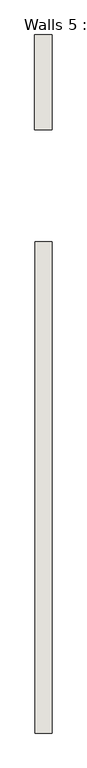
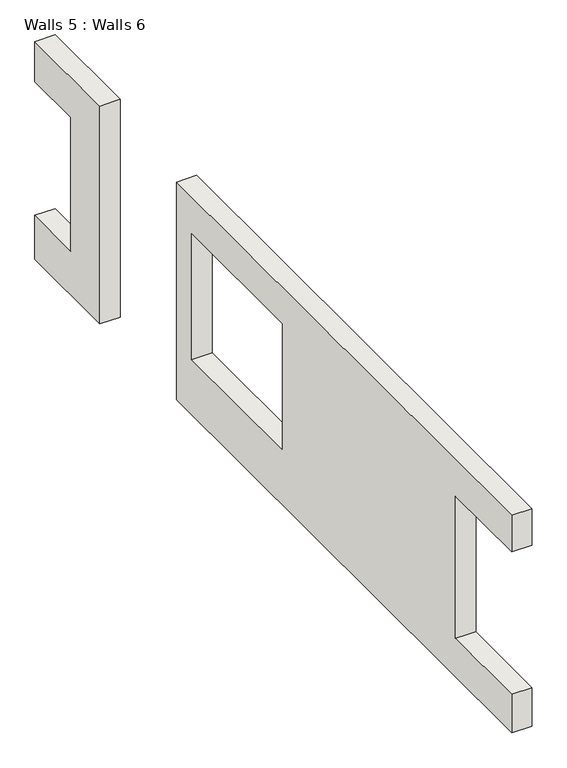
"""IFC4 building model written with IfcOpenShell, lengths in millimetres: wall geometry, Walls 5 : Walls 6."""

from ifc_helpers import new_model, si_unit, frame, origin, place, context, project, spatial, polyline, outline, extrude, source, transform, mapped, element, save


def walls_5_walls_6_e556a0bb(model_context):
    return source(origin(), model_context, "Body", "SweptSolid", [
        extrude(outline(polyline([(7992.6740933, 11277.6), (9929.9674246, 11277.6), (9929.9674246, 10551.6668798), (8863.1674246, 10551.6668798), (8863.1674246, 8113.2668798), (9929.9674246, 8113.2668798), (9929.9674246, 7315.2), (7992.6740933, 7315.2), (7992.6740933, 11277.6)])), frame((-9213.5370448, 0.0, 0.0), z_axis=(1.0, 0.0, 0.0), x_axis=(0.0, 1.0, 0.0)), (0.0, 0.0, 1.0), 352.9642709),
        extrude(outline(polyline([(5713.5674246, 11277.6), (5713.5674246, 7315.2), (-4294.0325754, 7315.2), (-4294.0325754, 8019.8696768), (-2617.6325754, 8019.8696768), (-2617.6325754, 10610.6696768), (-4294.0325754, 10610.6696768), (-4294.0325754, 11277.6), (5713.5674246, 11277.6)]), holes=[polyline([(2563.9674246, 10610.6696768), (2563.9674246, 8324.6696768), (5254.0047899, 8324.6696768), (5254.0047899, 10610.6696768), (2563.9674246, 10610.6696768)])]), frame((-9208.5505734, 0.0, 0.0), z_axis=(1.0, 0.0, 0.0), x_axis=(0.0, 1.0, 0.0)), (0.0, 0.0, 1.0), 347.9777995),
    ])


if __name__ == "__main__":
    model = new_model("IFC4")
    model_context = context("Model", 3, world=origin())
    ifc_project = project(units=[si_unit("LENGTHUNIT", "METRE", prefix="MILLI")], contexts=[model_context])
    site = spatial("IfcSite", under=ifc_project)
    building = spatial("IfcBuilding", under=site)
    placement = place(None, origin())
    walls_5_walls_6_shape = walls_5_walls_6_e556a0bb(model_context)
    element("IfcWall", 1, ObjectType="Walls 5 : Walls 6", at=placement, inside=building, context=model_context, shape_type="MappedRepresentation", body=[
        mapped(walls_5_walls_6_shape, transform((0.0, 0.0, 0.0), x_axis=(1.0, 0.0, 0.0), y_axis=(0.0, 1.0, 0.0), z_axis=(0.0, 0.0, 1.0))),
    ])
    save(model, "model.ifc")

# Revit data of these elements
# Element 1 (IfcWall, "Walls 5 : Walls 6")
#   Materials on its faces: "Default Wall"
# Materials
#   "Default Wall": colour RGB 128 128 128, transparency 0
